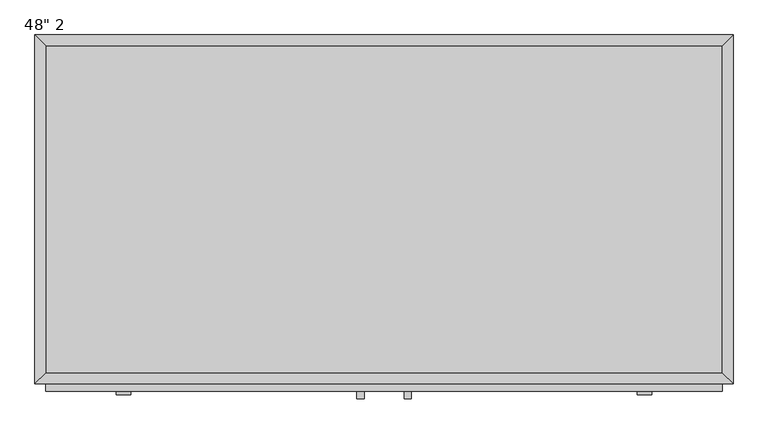
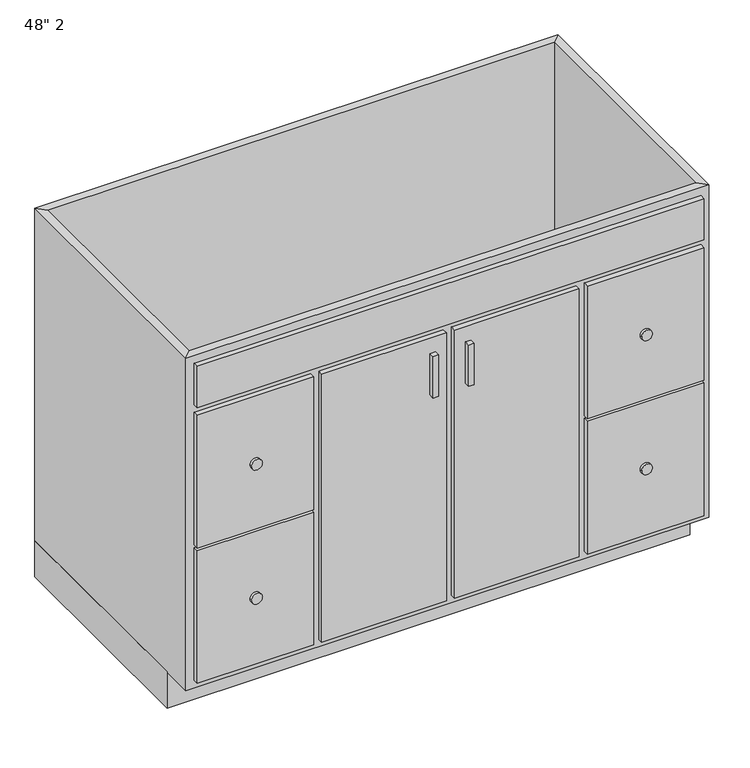
"""IFC4 building model written with IfcOpenShell, lengths in millimetres: furniture geometry."""

from ifc_helpers import new_model, si_unit, point, frame, frame_2d, origin, origin_with_axes, place, context, project, spatial, polyline, circle_curve, trimmed, segment, composite_curve, outline, extrude, faceted_brep, source, transform, mapped, element, save


def furniture_e236c193(model_context):
    return source(origin(), model_context, "Body", "SolidModel", [
        extrude(outline(polyline([(700.44496, 0.0), (700.44496, -533.4), (-518.75504, -533.4), (-518.75504, 0.0), (700.44496, 0.0)])), origin_with_axes(), (0.0, 0.0, 1.0), 88.9),
        faceted_brep([(681.39496, -590.55, 908.05), (681.39496, -590.55, 88.9), (-499.70504, -590.55, 88.9), (-499.70504, -590.55, 908.05), (700.44496, -609.6, 908.05), (-518.75504, -609.6, 908.05), (700.44496, -609.6, 88.9), (-518.75504, -609.6, 88.9), (-499.70504, -19.05, 88.9), (-499.70504, -19.05, 908.05), (-518.75504, 0.0, 908.05), (-518.75504, 0.0, 88.9), (681.39496, -19.05, 88.9), (681.39496, -19.05, 908.05), (700.44496, 0.0, 908.05), (700.44496, 0.0, 88.9)], [[[0, 1, 2, 3]], [[4, 0, 3, 5]], [[6, 4, 5, 7]], [[1, 6, 7, 2]], [[3, 2, 8, 9]], [[5, 3, 9, 10]], [[7, 5, 10, 11]], [[2, 7, 11, 8]], [[9, 8, 12, 13]], [[10, 9, 13, 14]], [[11, 10, 14, 15]], [[8, 11, 15, 12]], [[13, 12, 1, 0]], [[14, 13, 0, 4]], [[15, 14, 4, 6]], [[12, 15, 6, 1]]]),
        extrude(outline(polyline([(681.39496, -19.05), (681.39496, -590.55), (-499.70504, -590.55), (-499.70504, -19.05), (681.39496, -19.05)])), frame((0.0, 0.0, 88.9), z_axis=(0.0, 0.0, 1.0), x_axis=(1.0, 0.0, 0.0)), (0.0, 0.0, 1.0), 19.05),
        extrude(outline(composite_curve([segment(trimmed(circle_curve(frame_2d((273.05, 545.66371)), 12.7), [point((273.05, 532.96371))], [point((273.05, 558.36371))], False, "CARTESIAN"), True, "CONTINUOUS"), segment(trimmed(circle_curve(frame_2d((273.05, 545.66371)), 12.7), [point((273.05, 558.36371))], [point((273.05, 532.96371))], False, "CARTESIAN"), True, "CONTINUOUS")], self_intersect=False)), frame((0.0, -628.65, 0.0), z_axis=(0.0, 1.0, 0.0), x_axis=(0.0, 0.0, 1.0)), (0.0, 0.0, 1.0), 6.35),
        extrude(outline(composite_curve([segment(trimmed(circle_curve(frame_2d((603.25, 545.66371)), 12.7), [point((603.25, 532.96371))], [point((603.25, 558.36371))], False, "CARTESIAN"), True, "CONTINUOUS"), segment(trimmed(circle_curve(frame_2d((603.25, 545.66371)), 12.7), [point((603.25, 558.36371))], [point((603.25, 532.96371))], False, "CARTESIAN"), True, "CONTINUOUS")], self_intersect=False)), frame((0.0, -628.65, 0.0), z_axis=(0.0, 1.0, 0.0), x_axis=(0.0, 0.0, 1.0)), (0.0, 0.0, 1.0), 6.35),
        extrude(outline(composite_curve([segment(trimmed(circle_curve(frame_2d((603.25, -363.97379)), 12.7), [point((603.25, -376.67379))], [point((603.25, -351.27379))], False, "CARTESIAN"), True, "CONTINUOUS"), segment(trimmed(circle_curve(frame_2d((603.25, -363.97379)), 12.7), [point((603.25, -351.27379))], [point((603.25, -376.67379))], False, "CARTESIAN"), True, "CONTINUOUS")], self_intersect=False)), frame((0.0, -628.65, 0.0), z_axis=(0.0, 1.0, 0.0), x_axis=(0.0, 0.0, 1.0)), (0.0, 0.0, 1.0), 6.35),
        extrude(outline(composite_curve([segment(trimmed(circle_curve(frame_2d((273.05, -363.97379)), 12.7), [point((273.05, -376.67379))], [point((273.05, -351.27379))], False, "CARTESIAN"), True, "CONTINUOUS"), segment(trimmed(circle_curve(frame_2d((273.05, -363.97379)), 12.7), [point((273.05, -351.27379))], [point((273.05, -376.67379))], False, "CARTESIAN"), True, "CONTINUOUS")], self_intersect=False)), frame((0.0, -628.65, 0.0), z_axis=(0.0, 1.0, 0.0), x_axis=(0.0, 0.0, 1.0)), (0.0, 0.0, 1.0), 6.35),
        extrude(outline(polyline([(55.91996, -635.0), (43.21996, -635.0), (43.21996, -622.3), (55.91996, -622.3), (55.91996, -635.0)])), frame((0.0, 0.0, 628.65), z_axis=(0.0, 0.0, 1.0), x_axis=(1.0, 0.0, 0.0)), (0.0, 0.0, 1.0), 101.6),
        extrude(outline(polyline([(138.46996, -635.0), (125.76996, -635.0), (125.76996, -622.3), (138.46996, -622.3), (138.46996, -635.0)])), frame((0.0, 0.0, 628.65), z_axis=(0.0, 0.0, 1.0), x_axis=(1.0, 0.0, 0.0)), (0.0, 0.0, 1.0), 101.6),
        extrude(outline(polyline([(681.39496, -622.3), (-499.70504, -622.3), (-499.70504, -609.6), (681.39496, -609.6), (681.39496, -622.3)])), frame((0.0, 0.0, 787.4), z_axis=(0.0, 0.0, 1.0), x_axis=(1.0, 0.0, 0.0)), (0.0, 0.0, 1.0), 101.6),
        extrude(outline(polyline([(681.39496, -622.3), (409.93246, -622.3), (409.93246, -609.6), (681.39496, -609.6), (681.39496, -622.3)])), frame((0.0, 0.0, 441.325), z_axis=(0.0, 0.0, 1.0), x_axis=(1.0, 0.0, 0.0)), (0.0, 0.0, 1.0), 327.025),
        extrude(outline(polyline([(681.39496, -622.3), (409.93246, -622.3), (409.93246, -609.6), (681.39496, -609.6), (681.39496, -622.3)])), frame((0.0, 0.0, 107.95), z_axis=(0.0, 0.0, 1.0), x_axis=(1.0, 0.0, 0.0)), (0.0, 0.0, 1.0), 327.025),
        extrude(outline(polyline([(-228.24254, -622.3), (-499.70504, -622.3), (-499.70504, -609.6), (-228.24254, -609.6), (-228.24254, -622.3)])), frame((0.0, 0.0, 441.325), z_axis=(0.0, 0.0, 1.0), x_axis=(1.0, 0.0, 0.0)), (0.0, 0.0, 1.0), 327.025),
        extrude(outline(polyline([(-228.24254, -622.3), (-499.70504, -622.3), (-499.70504, -609.6), (-228.24254, -609.6), (-228.24254, -622.3)])), frame((0.0, 0.0, 107.95), z_axis=(0.0, 0.0, 1.0), x_axis=(1.0, 0.0, 0.0)), (0.0, 0.0, 1.0), 327.025),
        extrude(outline(polyline([(81.31996, -622.3), (-209.19254, -622.3), (-209.19254, -609.6), (81.31996, -609.6), (81.31996, -622.3)])), frame((0.0, 0.0, 107.95), z_axis=(0.0, 0.0, 1.0), x_axis=(1.0, 0.0, 0.0)), (0.0, 0.0, 1.0), 660.4),
        extrude(outline(polyline([(390.88246, -622.3), (100.36996, -622.3), (100.36996, -609.6), (390.88246, -609.6), (390.88246, -622.3)])), frame((0.0, 0.0, 107.95), z_axis=(0.0, 0.0, 1.0), x_axis=(1.0, 0.0, 0.0)), (0.0, 0.0, 1.0), 660.4),
    ])


if __name__ == "__main__":
    model = new_model("IFC4")
    model_context = context("Model", 3, world=origin())
    ifc_project = project(units=[si_unit("LENGTHUNIT", "METRE", prefix="MILLI")], contexts=[model_context])
    site = spatial("IfcSite", under=ifc_project)
    building = spatial("IfcBuilding", under=site)
    placement = place(None, origin())
    furniture_shape = furniture_e236c193(model_context)
    element("IfcFurniture", 1, ObjectType="48\" 2", at=placement, inside=building, context=model_context, shape_type="MappedRepresentation", body=[
        mapped(furniture_shape, transform((0.0, 0.0, 0.0), x_axis=(1.0, 0.0, 0.0), y_axis=(0.0, 1.0, 0.0), z_axis=(0.0, 0.0, 1.0))),
    ])
    save(model, "model.ifc")

# Revit data of these elements
# Type "48\" 2"
#   Assembly Code = "C1030410"
#   Depth = 2' - 0"
#   Height = 2' - 11 3/4"
#   Toe Depth = 0' - 3"
#   Toe Height = 0' - 3 1/2"
#   Width = 4' - 0"
#   Cabinet Material = none
#   Door/Drawer Material = none
#   Handle Material = Cabinets - Handles
#   Default Elevation = 0
# Element 1 (IfcFurniture, "48\" 2")
#   Materials on its faces: "Cabinets", "Cabinets - Handles"
# Materials
#   "Cabinets - Handles": colour RGB 57 57 57, transparency 0
#   "Cabinets": colour RGB 249 249 249, transparency 0
